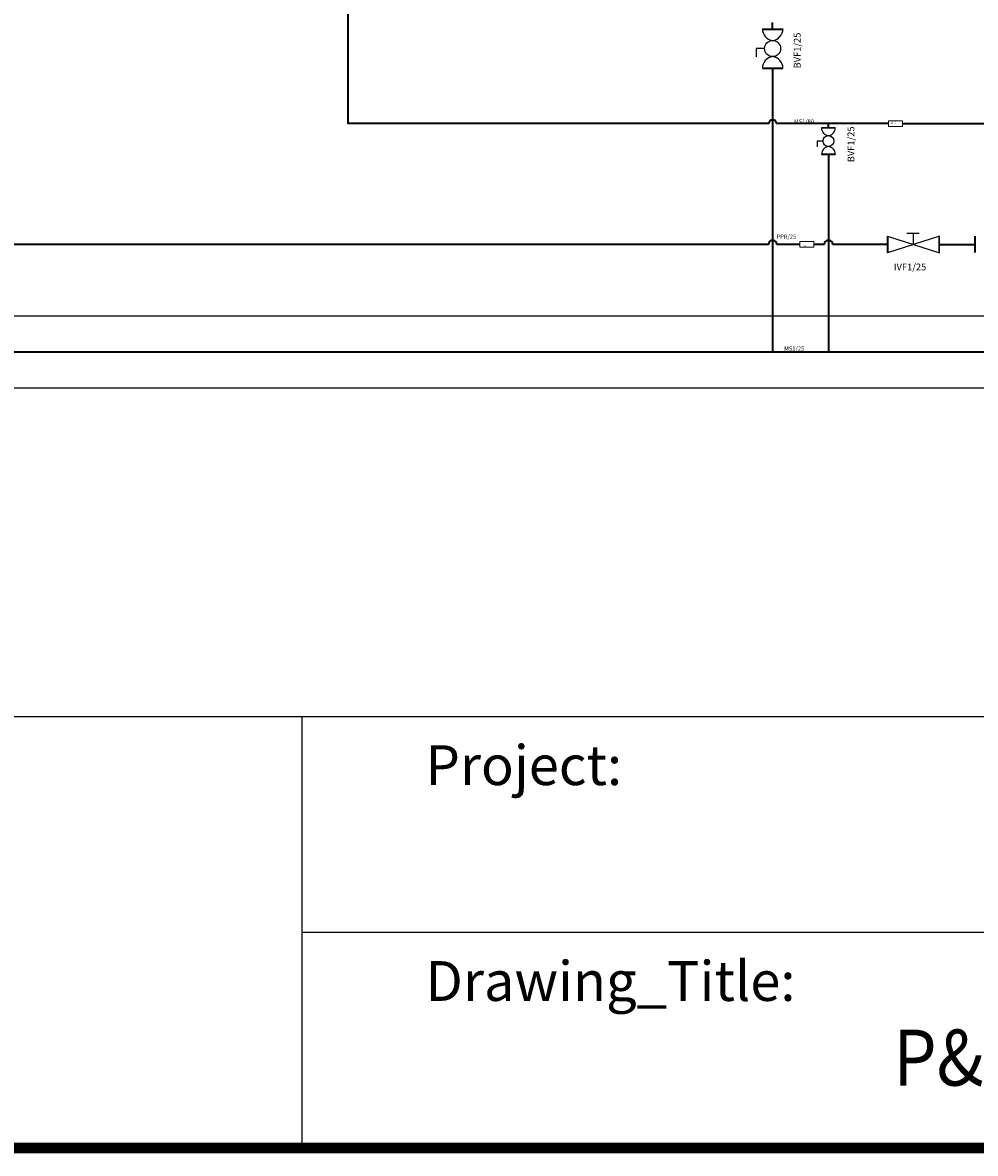
# Model space of a CAD drawing. Units: millimetres. Extents: x 353872 to 441597, y 126154 to 187356.
# Tile 2 of 28: x 367541 to 381210, y 126840 to 143050. Entities that reach past the tile are written whole.
import ezdxf

# ---------------------------------------------------------------- set-up
doc = ezdxf.new("R2010")
doc.units = ezdxf.units.MM
for name, color, linetype, lineweight in [('A-ANNO-DIMS', 2, 'Continuous', 18), ('P-ANNO-TEXT', 7, 'Continuous', 25), ('P-ANNO-TTLB', 7, 'Continuous', 25), ('P-INST-SIGN', 4, 'Continuous', 18), ('P-PIPE', 3, 'Continuous', 35), ('P-VALV', 2, 'Continuous', 25)]:
    doc.layers.add(name, color=color, linetype=linetype, lineweight=lineweight)
doc.styles.add('A1', font='ROMANT.shx', dxfattribs={"height": 200})
doc.styles.add('ROMANT', font='romant.shx', dxfattribs={"width": 0.8, "height": 3.5})
doc.styles.get("Standard").update_dxf_attribs({"font": 'arial.ttf'})
doc.dimstyles.get("Standard").update_dxf_attribs({"dimtxt": 0.18, "dimasz": 0.18, "dimexe": 0.18, "dimexo": 0.0625, "dimgap": 0.09, "dimtad": 0, "dimtih": 1, "dimtoh": 1, "dimdec": 4, "dimzin": 0, "dimdsep": 46, "dimtxsty": 'Standard', "dimcen": 0.09, "dimadec": 0, "dimazin": 0, "dimtfac": 1, "dimtdec": 4, "dimtofl": 0, "dimtmove": 0, "dimatfit": 3, "dimfxl": 1, "dimtolj": 1, "dimtzin": 0, "dimarcsym": 0})

# ---------------------------------------------------------------- blocks, each defined once
blk = doc.blocks.new('VALVE-E')
for points in [[(0, 7), (197, 7)], [(0, 5), (197, 4)], [(0, 2), (0, 0), (197, 0), (197, 3)], [(0, 2), (0, 2), (195, 2), (197, 2)]]:
    blk.add_lwpolyline(points)
for centre, start, end in [((113, 1), 97.3612, 180.5798), ((85, 2), 359.2193, 82.8397)]:
    blk.add_arc(centre, 113, start, end)
blk = doc.blocks.new('*D27')
at = {"layer": 'A-ANNO-DIMS', "color": 0, "lineweight": -2, "transparency": 16777216}
for p, q in [((366977, 138848), (440591, 138848)), ((440591, 138848), (440591, 138331)), ((440591, 137813), (440591, 138330)), ((366977, 137813), (440591, 137813))]:
    blk.add_line(p, q, dxfattribs=at)
at = {"layer": 'A-ANNO-DIMS', "color": 0, "transparency": 16777216}
for points in [[(440591, 138848), (440591, 138848), (440591, 138848)], [(440591, 137813), (440591, 137813), (440591, 137813)]]:
    blk.add_solid(points, dxfattribs=at)
at = {"layer": 'Defpoints', "color": 0, "transparency": 16777216}
for p in [(366977, 138848), (366977, 137813), (440591, 137813)]:
    blk.add_point(p, dxfattribs=at)
at = {"layer": 'A-ANNO-DIMS', "color": 0, "transparency": 16777216, "insert": (440591, 138330), "char_height": 0.18, "attachment_point": 5}
blk.add_mtext('\\A1;1035.2', dxfattribs=at)

msp = doc.modelspace()

# ---------------------------------------------------------------- linework, layer by layer
at = {"layer": 'P-ANNO-TTLB'}
for p, q in [((353948.03, 133103.92), (440835.19, 133103.92)), ((371550.6, 126916.34), (371550.6, 133103.92)), ((371550.6, 130010.13), (440835.19, 130010.13))]:
    msp.add_line(p, q, dxfattribs=at)
at = {"layer": 'P-ANNO-TTLB', "const_width": 152.43}
msp.add_lwpolyline([(353948.03, 187280.05), (353948.03, 126916.34), (440835.19, 126916.34), (440835.19, 187280.05)], close=True, dxfattribs=at)
at = {"layer": 'P-INST-SIGN'}
for points in [[(379961.46, 141642.67), (380161.54, 141642.67), (380161.54, 141561.54), (379961.46, 141561.54)], [(378690.5, 139911.03), (378890.59, 139911.03), (378890.59, 139829.9), (378690.5, 139829.9)]]:
    msp.add_lwpolyline(points, close=True, dxfattribs=at)
at = {"layer": 'P-PIPE'}
for p, q in [((378300.47, 142962.89), (378300.47, 143050.39)), ((378300.47, 142562.38), (378300.47, 142562.33)), ((378300.47, 142393.49), (378300.47, 138330.45)), ((379101.55, 141543.3), (379101.55, 141602.11)), ((379101.56, 141167.51), (379101.56, 138330.45)), ((381199.45, 139991.02), (381199.45, 139752.47)), ((380692.84, 139870.46), (381199.45, 139870.46)), ((366976.76, 138330.45), (381521.27, 138330.45))]:
    msp.add_line(p, q, dxfattribs=at)
for points in [[(379961.46, 141602.11), (378356.61, 141602.11, 1), (378244.32, 141602.11), (372209.04, 141602.11), (372209.04, 146769.18)], [(378690.5, 139870.46), (378361.72, 139870.46, 0.99121811), (378239.22, 139870.46), (366976.76, 139870.46)], [(379948.81, 139870.46), (379162.81, 139870.46, 0.99121811), (379040.31, 139870.46), (378890.59, 139870.46)]]:
    msp.add_lwpolyline(points, format="xyb", dxfattribs=at)
msp.add_lwpolyline([(380161.54, 141602.11), (389676.87, 141602.11), (389676.87, 140682.39), (392361.87, 140682.39), (392361.87, 141110.07)], dxfattribs=at)
at = {"layer": 'P-VALV'}
for p, q in [((380224.82, 140034.39), (380401.04, 140034.39)), ((380320.83, 139870.46), (380320.83, 140034.39))]:
    msp.add_line(p, q, dxfattribs=at)
for points in [[(378153.54, 142959.48), (378153.54, 142962.89), (378447.4, 142962.89), (378447.4, 142958.32)], [(378153.54, 142959.64), (378156.84, 142959.6), (378444.1, 142959.6), (378447.41, 142959.58)], [(378153.61, 142956.17), (378447.36, 142956.3)], [(378153.74, 142952.71), (378447.22, 142952.64)], [(378184.27, 142678.19), (378063.01, 142678.19), (378063.01, 142559.13)], [(378153.54, 142396.9), (378153.54, 142393.49), (378447.4, 142393.49), (378447.4, 142398.06)], [(378153.54, 142396.81), (378153.54, 142396.81), (378444.1, 142396.78), (378447.4, 142396.78)], [(378153.61, 142400.2), (378447.35, 142400.14)], [(378153.74, 142403.66), (378447.22, 142403.74)], [(379023.46, 141351.97), (378941.97, 141351.97), (378941.97, 141271.96)], [(379956.72, 139752.47), (379956.72, 139988.45)], [(380684.93, 139988.45), (380684.93, 139752.47)]]:
    msp.add_lwpolyline(points, dxfattribs=at)
msp.add_lwpolyline([(380692.84, 139749.91), (380692.84, 139991.02), (379948.81, 139749.91), (379948.81, 139991.02)], close=True, dxfattribs=at)
for centre, radius in [((378300.08, 142678.19), 115.81), ((379101.28, 141351.97), 77.83)]:
    msp.add_circle(centre, radius, dxfattribs=at)
for centre, radius, start, end in [((378322.06, 142961.19), 168.53, 179.420152, 262.638767), ((378279.54, 142960.6), 167.87, 277.160335, 0.780747), ((378322.06, 142395.19), 168.53, 97.361233, 180.579848), ((378279.54, 142395.77), 167.87, 359.219253, 82.839665)]:
    msp.add_arc(centre, radius, start, end, dxfattribs=at)

# ---------------------------------------------------------------- block references
at = {"layer": 'P-VALV', "rotation": 181.3019170019436}
msp.add_blockref('VALVE-E', (379199.86, 141545.55), dxfattribs=at)
at = {"layer": 'P-VALV'}
msp.add_blockref('VALVE-E', (379002.8, 141160.64), dxfattribs=at)

# ---------------------------------------------------------------- texts
at = {"layer": 'P-ANNO-TEXT'}
for p in [(378701.94, 142393.49), (379473, 141048.24)]:
    msp.add_text('BVF1/25', height=98.09, rotation=90, dxfattribs=at).set_placement(p)
for s, height, p in [('MS1/80', 60.86, (378606.13, 141602.11)), ('1HC', 26.582, (380000.34, 141602.11)), ('PPR/25', 60.86, (378356.48, 139951.03)), ('1H', 26.582, (378730.97, 139829.9)), ('IVF1/25', 98.09, (380039.49, 139497.91)), ('MS1/25', 60.86, (378466.32, 138347.78))]:
    msp.add_text(s, height=height, dxfattribs=at).set_placement(p)
at = {"layer": 'P-ANNO-TEXT', "style": 'ROMANT', "width": 0.9}
msp.add_text('P&ID SSR 6.0KL REACTOR', height=802.0939, dxfattribs=at).set_placement((380031.07, 127811.87))
at = {"layer": 'P-ANNO-TTLB', "style": 'A1'}
for s, height, p in [('Project:', 570.687, (373321.52, 132119.64)), ('Drawing_Title:', 570.6871, (373321.52, 129025.85))]:
    msp.add_text(s, height=height, dxfattribs=at).set_placement(p)

# ---------------------------------------------------------------- dimensions: what is measured, and where the dimension line sits
at = {"layer": 'A-ANNO-DIMS'}
dim = msp.add_linear_dim(base=(440591, 137812.84), p1=(366976.76, 138848.06), p2=(366976.76, 137812.84), angle=90, dimstyle='Standard', override={"dimdec": 1, "dimlfac": 1, "dimrnd": 0, "dimzin": 0, "dimdsep": 46, "dimlunit": 2}, dxfattribs=at)
dim.commit()
dim.dimension.update_dxf_attribs({"geometry": '*D27', "text_midpoint": (440591, 138330.45)})

doc.saveas('drawing.dxf')
